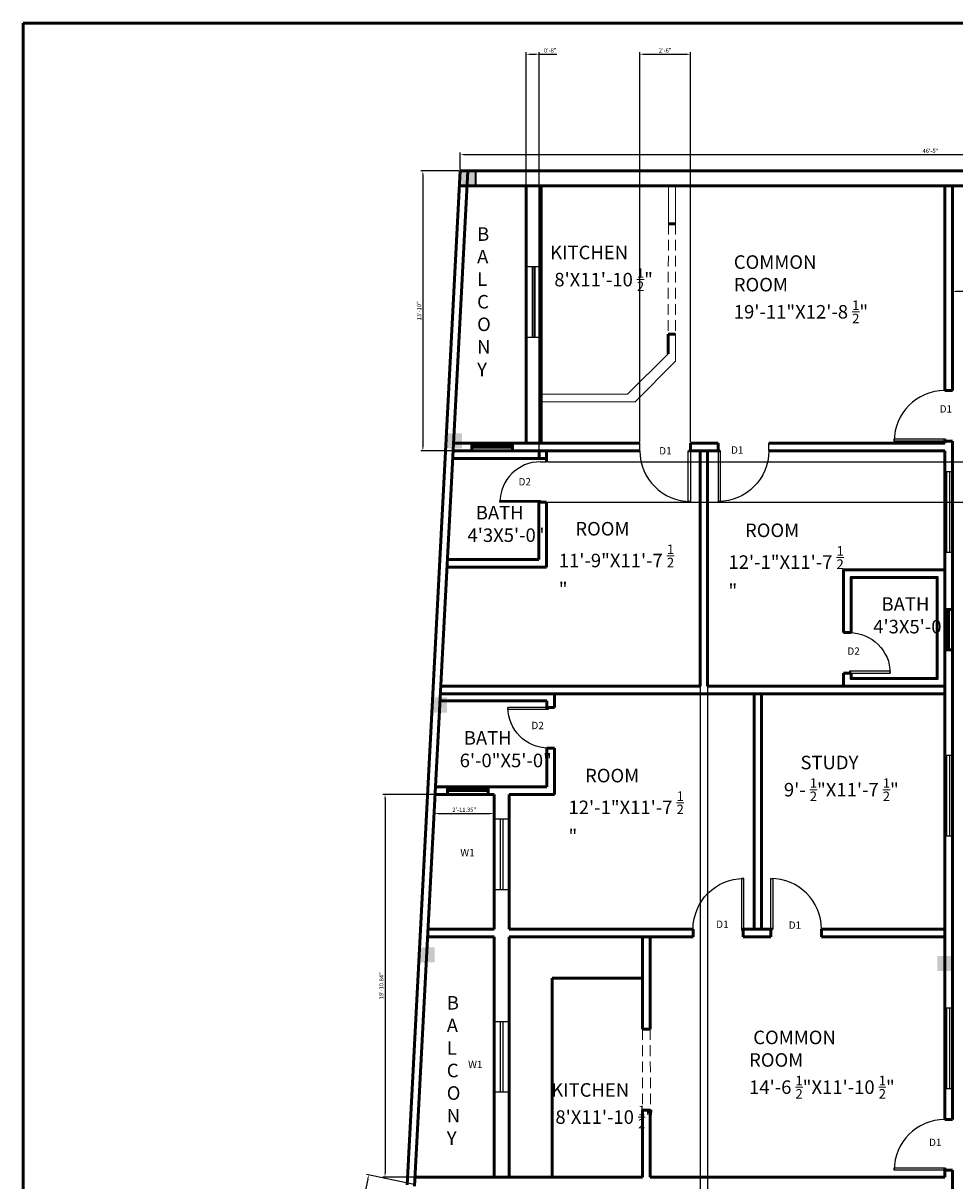
# Model space of a CAD drawing. Units: millimetres. Extents: x 1945 to 2943, y 628 to 2340.
# Tile 4 of 5: x 1945 to 2497, y 1654 to 2340. Entities that reach past the tile are written whole.
import ezdxf

# ---------------------------------------------------------------- set-up
doc = ezdxf.new("R2010")
doc.units = ezdxf.units.MM
doc.linetypes.add('DASHED', pattern=[19.05, 12.7, -6.35])
for name, color, linetype, lineweight in [('A-ANNO-DIMS', 2, 'Continuous', 18), ('A-ANNO-TEXT', 7, 'Continuous', 18), ('A-AREA-IDEN', 3, 'Continuous', 18), ('A-COLS', 1, 'Continuous', 35), ('A-DOOR', 4, 'Continuous', 25), ('A-FLOR-FIXT', 8, 'Continuous', 18), ('A-GLAZ', 4, 'Continuous', 25), ('A-WALL', 7, 'Continuous', 50), ('A-WALL-OPNG', 8, 'DASHED', 18)]:
    doc.layers.add(name, color=color, linetype=linetype, lineweight=lineweight)
doc.styles.get("Standard").update_dxf_attribs({"font": 'arial.ttf'})
doc.styles.add('YQ_DIM', font='SUPEROS.SHX', dxfattribs={"width": 0.8, "bigfont": 'HZDX.SHX'})
doc.dimstyles.new('ISO-25', dxfattribs={"dimtxt": 2.5, "dimasz": 2.5, "dimexe": 1.25, "dimexo": 0.625, "dimtad": 1, "dimlunit": 3, "dimtxsty": 'Standard', "dimcen": 2.5, "dimadec": 0, "dimazin": 0, "dimtfac": 1, "dimtmove": 0, "dimatfit": 3, "dimfxl": 1, "dimarcsym": 0})

# ---------------------------------------------------------------- blocks, each defined once
blk = doc.blocks.new('*U3')
for p, q in [((0, 0), (0, -6)), ((40, 0), (40, -6))]:
    blk.add_line(p, q)
blk.add_lwpolyline([(0, 0), (0, 40), (1.75, 40), (1.75, 0)], close=True)
blk.add_arc((0, 0), 40, 0, 90)
blk = doc.blocks.new('*D7')
at = {"layer": 'A-ANNO-DIMS', "color": 0, "lineweight": -2, "ltscale": 0.5, "transparency": 16777216}
for p, q in [((2495.1, 2172.25), (2495.1, 2182.39)), ((2633.6, 2172.25), (2633.6, 2182.39)), ((2631.1, 2181.14), (2497.6, 2181.14))]:
    blk.add_line(p, q, dxfattribs=at)
at = {"layer": 'A-ANNO-DIMS', "color": 0, "ltscale": 0.5, "transparency": 16777216}
for points in [[(2497.6, 2181.56), (2497.6, 2180.72), (2495.1, 2181.14)], [(2631.1, 2181.56), (2631.1, 2180.72), (2633.6, 2181.14)]]:
    blk.add_solid(points, dxfattribs=at)
at = {"layer": 'Defpoints', "color": 0, "ltscale": 0.5, "transparency": 16777216}
for p in [(2495.1, 2181.14), (2495.1, 2171.62), (2633.6, 2171.62)]:
    blk.add_point(p, dxfattribs=at)
at = {"layer": 'A-ANNO-DIMS', "color": 0, "ltscale": 0.5, "transparency": 16777216, "insert": (2564.35, 2183.04), "char_height": 2.5, "attachment_point": 5}
blk.add_mtext('11\'-6.5"', dxfattribs=at)
blk = doc.blocks.new('*D8')
at = {"layer": 'A-ANNO-DIMS', "color": 0, "lineweight": -2, "ltscale": 0.5, "transparency": 16777216}
for p, q in [((2202.97, 2252.62), (2180.19, 2252.62)), ((2181.44, 2250.12), (2181.44, 2089.12)), ((2198.78, 2086.62), (2180.19, 2086.62))]:
    blk.add_line(p, q, dxfattribs=at)
at = {"layer": 'A-ANNO-DIMS', "color": 0, "ltscale": 0.5, "transparency": 16777216}
for points in [[(2181.02, 2250.12), (2181.85, 2250.12), (2181.44, 2252.62)], [(2181.02, 2089.12), (2181.85, 2089.12), (2181.44, 2086.62)]]:
    blk.add_solid(points, dxfattribs=at)
at = {"layer": 'Defpoints', "color": 0, "ltscale": 0.5, "transparency": 16777216}
for p in [(2203.6, 2252.62), (2181.44, 2086.62), (2199.4, 2086.62)]:
    blk.add_point(p, dxfattribs=at)
at = {"layer": 'A-ANNO-DIMS', "color": 0, "ltscale": 0.5, "transparency": 16777216, "insert": (2179.54, 2169.62), "char_height": 2.5, "attachment_point": 5, "rotation": 90}
blk.add_mtext('13\'-10"', dxfattribs=at)
blk = doc.blocks.new('*D9')
at = {"layer": 'A-ANNO-DIMS', "color": 0, "lineweight": -2, "ltscale": 0.5, "transparency": 16777216}
for p, q in [((2188.11, 1882.96), (2157.79, 1882.96)), ((2159.04, 1880.46), (2159.04, 1658.62)), ((2176.22, 1656.12), (2157.79, 1656.12))]:
    blk.add_line(p, q, dxfattribs=at)
at = {"layer": 'A-ANNO-DIMS', "color": 0, "ltscale": 0.5, "transparency": 16777216}
for points in [[(2158.62, 1880.46), (2159.45, 1880.46), (2159.04, 1882.96)], [(2158.62, 1658.62), (2159.45, 1658.62), (2159.04, 1656.12)]]:
    blk.add_solid(points, dxfattribs=at)
at = {"layer": 'Defpoints', "color": 0, "ltscale": 0.5, "transparency": 16777216}
for p in [(2188.73, 1882.96), (2159.04, 1656.12), (2176.84, 1656.12)]:
    blk.add_point(p, dxfattribs=at)
at = {"layer": 'A-ANNO-DIMS', "color": 0, "ltscale": 0.5, "transparency": 16777216, "insert": (2157.14, 1769.54), "char_height": 2.5, "attachment_point": 5, "rotation": 90}
blk.add_mtext('18\'-10.84"', dxfattribs=at)
blk = doc.blocks.new('*D10')
at = {"layer": 'A-ANNO-DIMS', "color": 0, "lineweight": -2, "ltscale": 0.5, "transparency": 16777216}
for p, q in [((2148.79, 1654.96), (2010, 994.38)), ((2176.25, 1651.75), (2148.08, 1657.67)), ((2036.43, 986.28), (2008.27, 992.19))]:
    blk.add_line(p, q, dxfattribs=at)
at = {"layer": 'A-ANNO-DIMS', "color": 0, "ltscale": 0.5, "transparency": 16777216}
for points in [[(2148.39, 1655.05), (2149.2, 1654.88), (2149.31, 1657.41)], [(2009.6, 994.47), (2010.41, 994.3), (2009.49, 991.94)]]:
    blk.add_solid(points, dxfattribs=at)
at = {"layer": 'Defpoints', "color": 0, "ltscale": 0.5, "transparency": 16777216}
for p in [(2176.86, 1651.62), (2009.49, 991.94), (2037.04, 986.15)]:
    blk.add_point(p, dxfattribs=at)
at = {"layer": 'A-ANNO-DIMS', "color": 0, "ltscale": 0.5, "transparency": 16777216, "insert": (2077.54, 1325.06), "char_height": 2.5, "attachment_point": 5, "rotation": 78.13463}
blk.add_mtext('56\'-8"', dxfattribs=at)
blk = doc.blocks.new('*D11')
at = {"layer": 'A-ANNO-DIMS', "color": 0, "lineweight": -2, "ltscale": 0.5, "transparency": 16777216}
for p, q in [((2188.24, 1873.05), (2188.24, 1870.37)), ((2190.74, 1871.62), (2221.1, 1871.62)), ((2223.6, 1873.05), (2223.6, 1870.37))]:
    blk.add_line(p, q, dxfattribs=at)
at = {"layer": 'A-ANNO-DIMS', "color": 0, "ltscale": 0.5, "transparency": 16777216}
for points in [[(2190.74, 1872.03), (2190.74, 1871.2), (2188.24, 1871.62)], [(2221.1, 1872.03), (2221.1, 1871.2), (2223.6, 1871.62)]]:
    blk.add_solid(points, dxfattribs=at)
at = {"layer": 'Defpoints', "color": 0, "ltscale": 0.5, "transparency": 16777216}
for p in [(2188.24, 1873.68), (2223.6, 1873.68), (2223.6, 1871.62)]:
    blk.add_point(p, dxfattribs=at)
at = {"layer": 'A-ANNO-DIMS', "color": 0, "ltscale": 0.5, "transparency": 16777216, "insert": (2205.92, 1873.52), "char_height": 2.5, "attachment_point": 5}
blk.add_mtext('2\'-11.35"', dxfattribs=at)
blk = doc.blocks.new('*D17')
at = {"layer": 'A-ANNO-DIMS', "color": 0, "lineweight": -2, "transparency": 16777216}
for p, q in [((2203.6, 2253.25), (2203.6, 2263.48)), ((2206.1, 2262.23), (2758.1, 2262.23)), ((2760.6, 2253.25), (2760.6, 2263.48))]:
    blk.add_line(p, q, dxfattribs=at)
at = {"layer": 'A-ANNO-DIMS', "color": 0, "transparency": 16777216}
for points in [[(2206.1, 2262.64), (2206.1, 2261.81), (2203.6, 2262.23)], [(2758.1, 2262.64), (2758.1, 2261.81), (2760.6, 2262.23)]]:
    blk.add_solid(points, dxfattribs=at)
at = {"layer": 'Defpoints', "color": 0, "transparency": 16777216}
for p in [(2760.6, 2262.23), (2203.6, 2252.62), (2760.6, 2252.62)]:
    blk.add_point(p, dxfattribs=at)
at = {"layer": 'A-ANNO-DIMS', "color": 0, "transparency": 16777216, "insert": (2482.1, 2264.13), "char_height": 2.5, "attachment_point": 5}
blk.add_mtext('46\'-5"', dxfattribs=at)
blk = doc.blocks.new('WIN-W1')
for points in [[(0, 48), (4.5, 48), (4.5, 0), (0, 0)], [(1.29, 48), (2.82, 48), (2.82, 0), (1.29, 0)]]:
    blk.add_lwpolyline(points, close=True)
blk = doc.blocks.new('WIN-W2')
for points in [[(0, 42), (9, 42), (9, 0), (0, 0)], [(3.84, 42), (5.13, 42), (5.13, 0), (3.84, 0)]]:
    blk.add_lwpolyline(points, close=True)
blk = doc.blocks.new('*D27')
at = {"layer": 'A-ANNO-DIMS', "color": 0, "lineweight": -2, "transparency": 16777216}
for p, q in [((2309.97, 2091.75), (2309.97, 2322.97)), ((2312.47, 2321.72), (2337.47, 2321.72)), ((2339.97, 2091.75), (2339.97, 2322.97))]:
    blk.add_line(p, q, dxfattribs=at)
at = {"layer": 'A-ANNO-DIMS', "color": 0, "transparency": 16777216}
for points in [[(2312.47, 2322.14), (2312.47, 2321.3), (2309.97, 2321.72)], [(2337.47, 2322.14), (2337.47, 2321.3), (2339.97, 2321.72)]]:
    blk.add_solid(points, dxfattribs=at)
at = {"layer": 'Defpoints', "color": 0, "transparency": 16777216}
for p in [(2339.97, 2321.72), (2309.97, 2091.12), (2339.97, 2091.12)]:
    blk.add_point(p, dxfattribs=at)
at = {"layer": 'A-ANNO-DIMS', "color": 0, "transparency": 16777216, "insert": (2324.97, 2323.62), "char_height": 2.5, "attachment_point": 5}
blk.add_mtext('2\'-6"', dxfattribs=at)
blk = doc.blocks.new('*D28')
at = {"layer": 'A-ANNO-DIMS', "color": 0, "lineweight": -2, "transparency": 16777216}
for p, q in [((2255.29, 2080.13), (2830.95, 2080.13)), ((2829.7, 2058.63), (2829.7, 2077.63)), ((2255.29, 2056.13), (2830.95, 2056.13))]:
    blk.add_line(p, q, dxfattribs=at)
at = {"layer": 'A-ANNO-DIMS', "color": 0, "transparency": 16777216}
for points in [[(2829.28, 2077.63), (2830.11, 2077.63), (2829.7, 2080.13)], [(2829.28, 2058.63), (2830.11, 2058.63), (2829.7, 2056.13)]]:
    blk.add_solid(points, dxfattribs=at)
at = {"layer": 'Defpoints', "color": 0, "transparency": 16777216}
for p in [(2254.67, 2080.13), (2829.7, 2080.13), (2254.67, 2056.13)]:
    blk.add_point(p, dxfattribs=at)
at = {"layer": 'A-ANNO-DIMS', "color": 0, "transparency": 16777216, "insert": (2827.8, 2068.13), "char_height": 2.5, "attachment_point": 5, "rotation": 90}
blk.add_mtext('2\'-0"', dxfattribs=at)
blk = doc.blocks.new('*D29')
at = {"layer": 'A-ANNO-DIMS', "color": 0, "lineweight": -2, "transparency": 16777216}
for p, q in [((2242.6, 2091.75), (2242.6, 2322.97)), ((2245.1, 2321.72), (2247.9, 2321.72)), ((2250.4, 2087.25), (2250.4, 2322.97)), ((2250.4, 2321.72), (2260.8, 2321.72))]:
    blk.add_line(p, q, dxfattribs=at)
at = {"layer": 'A-ANNO-DIMS', "color": 0, "transparency": 16777216}
for points in [[(2245.1, 2322.14), (2245.1, 2321.3), (2242.6, 2321.72)], [(2247.9, 2322.14), (2247.9, 2321.3), (2250.4, 2321.72)]]:
    blk.add_solid(points, dxfattribs=at)
at = {"layer": 'Defpoints', "color": 0, "transparency": 16777216}
for p in [(2250.4, 2321.72), (2242.6, 2091.12), (2250.4, 2086.62)]:
    blk.add_point(p, dxfattribs=at)
at = {"layer": 'A-ANNO-DIMS', "color": 0, "transparency": 16777216, "insert": (2256.85, 2323.62), "char_height": 2.5, "attachment_point": 5}
blk.add_mtext('0\'-8"', dxfattribs=at)
blk = doc.blocks.new('*D30')
at = {"layer": 'A-ANNO-DIMS', "color": 0, "lineweight": -2, "transparency": 16777216}
for p, q in [((2345.6, 2086), (2345.6, 856.56)), ((2350.1, 2086), (2350.1, 856.56)), ((2343.1, 857.81), (2340.6, 857.81)), ((2345.6, 857.81), (2350.1, 857.81)), ((2352.6, 857.81), (2368.82, 857.81))]:
    blk.add_line(p, q, dxfattribs=at)
at = {"layer": 'A-ANNO-DIMS', "color": 0, "transparency": 16777216}
for points in [[(2343.1, 858.23), (2343.1, 857.39), (2345.6, 857.81)], [(2352.6, 858.23), (2352.6, 857.39), (2350.1, 857.81)]]:
    blk.add_solid(points, dxfattribs=at)
at = {"layer": 'Defpoints', "color": 0, "transparency": 16777216}
for p in [(2345.6, 2086.62), (2350.1, 2086.62), (2350.1, 857.81)]:
    blk.add_point(p, dxfattribs=at)
at = {"layer": 'A-ANNO-DIMS', "color": 0, "transparency": 16777216, "insert": (2361.96, 859.73), "char_height": 2.5, "attachment_point": 5}
blk.add_mtext('0\'-4 1/2"', dxfattribs=at)

msp = doc.modelspace()

# ---------------------------------------------------------------- hatches: boundary and pattern name
at = {"layer": 'A-COLS'}
h = msp.add_hatch(color=256, dxfattribs=at)
h.dxf.hatch_style = 1
h.paths.add_polyline_path([(2212.597, 2252.621), (2203.597, 2252.621), (2203.597, 2243.621), (2212.597, 2243.621)])
h = msp.add_hatch(color=256, dxfattribs=at)
h.dxf.hatch_style = 1
h.paths.add_polyline_path([(2212.597, 2243.621), (2212.597, 2252.621), (2203.597, 2252.621), (2203.597, 2243.621)])
h = msp.add_hatch(color=256, dxfattribs=at)
h.dxf.hatch_style = 1
h.paths.add_polyline_path([(2212.597, 2243.621), (2212.597, 2252.621), (2203.597, 2252.621), (2203.597, 2243.621)])
h = msp.add_hatch(color=256, dxfattribs=at)
h.dxf.hatch_style = 1
h.paths.add_polyline_path([(2212.597, 2243.621), (2212.597, 2252.621), (2203.597, 2252.621), (2203.597, 2243.621)])
h = msp.add_hatch(color=256, dxfattribs=at)
h.dxf.hatch_style = 1
h.paths.add_polyline_path([(2212.597, 2243.621), (2212.597, 2252.621), (2203.597, 2252.621), (2203.597, 2243.621)])
h = msp.add_hatch(color=256, dxfattribs=at)
h.dxf.hatch_style = 1
h.paths.add_polyline_path([(2212.597, 2243.621), (2212.597, 2252.621), (2203.597, 2252.621), (2203.597, 2243.621)])
h = msp.add_hatch(color=256, dxfattribs=at)
h.dxf.hatch_style = 1
h.paths.add_polyline_path([(2212.597, 2243.621), (2212.597, 2252.621), (2203.597, 2252.621), (2203.597, 2243.621)])
h = msp.add_hatch(color=256, dxfattribs=at)
h.dxf.hatch_style = 1
h.paths.add_polyline_path([(2212.597, 2243.621), (2212.597, 2252.621), (2203.597, 2252.621), (2203.597, 2243.621)])
h = msp.add_hatch(color=256, dxfattribs=at)
h.dxf.hatch_style = 1
h.paths.add_polyline_path([(2212.597, 2243.621), (2212.597, 2252.621), (2203.597, 2252.621), (2203.597, 2243.621)])
h = msp.add_hatch(color=256, dxfattribs=at)
h.dxf.hatch_style = 1
h.paths.add_polyline_path([(2212.597, 2243.621), (2212.597, 2252.621), (2203.597, 2252.621), (2203.597, 2243.621)])
h = msp.add_hatch(color=256, dxfattribs=at)
h.dxf.hatch_style = 1
h.paths.add_polyline_path([(2212.597, 2243.621), (2212.597, 2252.621), (2203.597, 2252.621), (2203.597, 2243.621)])
h = msp.add_hatch(color=256, dxfattribs=at)
h.dxf.hatch_style = 1
h.paths.add_polyline_path([(2212.597, 2243.621), (2212.597, 2252.621), (2203.597, 2252.621), (2203.597, 2243.621)])
h = msp.add_hatch(color=256, dxfattribs=at)
h.dxf.hatch_style = 1
h.paths.add_polyline_path([(2212.597, 2243.621), (2212.597, 2252.621), (2203.597, 2252.621), (2203.597, 2243.621)])
h = msp.add_hatch(color=256, dxfattribs=at)
h.dxf.hatch_style = 1
h.paths.add_polyline_path([(2212.597, 2243.621), (2212.597, 2252.621), (2203.597, 2252.621), (2203.597, 2243.621)])
h = msp.add_hatch(color=256, dxfattribs=at)
h.dxf.hatch_style = 1
h.paths.add_polyline_path([(2212.597, 2243.621), (2212.597, 2252.621), (2203.597, 2252.621), (2203.597, 2243.621)])
h = msp.add_hatch(color=256, dxfattribs=at)
h.dxf.hatch_style = 1
h.paths.add_polyline_path([(2212.597, 2243.621), (2212.597, 2252.621), (2203.597, 2252.621), (2203.597, 2243.621)])
h = msp.add_hatch(color=256, dxfattribs=at)
h.dxf.hatch_style = 1
h.paths.add_polyline_path([(2212.597, 2243.621), (2212.597, 2252.621), (2203.597, 2252.621), (2203.597, 2243.621)])
h = msp.add_hatch(color=256, dxfattribs=at)
h.dxf.hatch_style = 1
h.paths.add_polyline_path([(2212.597, 2243.621), (2212.597, 2252.621), (2203.597, 2252.621), (2203.597, 2243.621)])
h = msp.add_hatch(color=256, dxfattribs=at)
h.dxf.hatch_style = 1
h.paths.add_polyline_path([(2204.673, 2097.037), (2195.673, 2097.037), (2195.673, 2088.037), (2204.673, 2088.037)])
h = msp.add_hatch(color=256, dxfattribs=at)
h.dxf.hatch_style = 1
h.paths.add_polyline_path([(2195.693, 1940.478), (2186.693, 1940.478), (2186.693, 1931.478), (2195.693, 1931.478)])
h = msp.add_hatch(color=256, dxfattribs=at)
h.dxf.hatch_style = 1
h.paths.add_polyline_path([(2188.404, 1792.332), (2179.404, 1792.332), (2179.404, 1783.332), (2188.404, 1783.332)])
h = msp.add_hatch(color=256, dxfattribs=at)
h.dxf.hatch_style = 1
h.paths.add_polyline_path([(2495.097, 1787.253), (2486.097, 1787.253), (2486.097, 1778.253), (2495.097, 1778.253)])

# ---------------------------------------------------------------- linework, layer by layer
msp.add_lwpolyline([(2203.597, 2252.621), (2212.597, 2252.621), (2212.597, 2243.621), (2203.597, 2243.621)], close=True, dxfattribs=at)
at = {"layer": 'A-FLOR-FIXT'}
for points in [[(2326.669, 2144.192), (2302.597, 2120.192), (2251.597, 2120.192), (2251.967, 2243.621), (2326.967, 2243.621), (2326.9, 2221.255)], [(2331.097, 2243.621), (2331.097, 2221.255)], [(2247.097, 2153.851), (2247.097, 2195.851)], [(2331.097, 2155.773), (2331.097, 2139.692), (2307.097, 2115.692), (2251.597, 2115.692)]]:
    msp.add_lwpolyline(points, dxfattribs=at)
at = {"layer": 'A-WALL'}
for p, q in [((2203.597, 2252.621), (2172.098, 1651.581)), ((2208.091, 2252.386), (2176.56, 1650.732)), ((2760.597, 2252.621), (2203.597, 2252.621)), ((2751.597, 2243.621), (2203.597, 2243.621)), ((2242.597, 2243.192), (2242.597, 2091.121)), ((2251.597, 2243.192), (2251.597, 2091.121)), ((2490.597, 2243.621), (2490.597, 2122.348)), ((2495.097, 2243.621), (2495.097, 2122.348)), ((2326.9, 2221.255), (2331.097, 2221.255)), ((2326.669, 2144.192), (2326.704, 2155.773)), ((2326.704, 2155.773), (2331.097, 2155.773)), ((2495.097, 2122.348), (2490.597, 2122.348)), ((2490.597, 2093.66), (2490.597, 2091.121)), ((2309.97, 2086.621), (2199.404, 2086.621)), ((2199.404, 2086.621), (2254.668, 2086.621)), ((2309.97, 2091.121), (2199.64, 2091.121)), ((2250.404, 2086.621), (2250.404, 2082.121)), ((2254.668, 2086.621), (2254.668, 2080.13)), ((2357.406, 2086.621), (2338.92, 2086.621)), ((2356.356, 2091.121), (2339.97, 2091.121)), ((2339.97, 2091.121), (2339.97, 2086.621)), ((2345.597, 2086.621), (2345.597, 1947.121)), ((2350.097, 2086.621), (2350.097, 1947.121)), ((2356.356, 2091.121), (2356.356, 2086.621)), ((2490.597, 2091.121), (2386.356, 2091.121)), ((2490.597, 2086.621), (2386.356, 2086.621)), ((2490.597, 2092.348), (2495.097, 2092.348)), ((2490.597, 2086.621), (2490.597, 1690.225)), ((2495.097, 2092.348), (2495.097, 1690.225)), ((2199.168, 2082.121), (2254.668, 2082.121)), ((2250.168, 2057.18), (2250.168, 2022.121)), ((2250.168, 2056.13), (2254.668, 2056.13)), ((2254.668, 2056.13), (2254.668, 2017.621)), ((2254.668, 2017.621), (2195.788, 2017.621)), ((2250.168, 2022.121), (2196.024, 2022.121)), ((2430.597, 1978.881), (2435.097, 1978.864)), ((2430.597, 1954.881), (2435.097, 1954.881)), ((2490.597, 1942.621), (2191.857, 1942.621)), ((2345.597, 1947.121), (2192.093, 1947.121)), ((2259.369, 1942.621), (2259.369, 1934.461)), ((2490.597, 1947.121), (2350.097, 1947.121)), ((2377.597, 1942.621), (2377.597, 1803.121)), ((2382.097, 1942.621), (2382.097, 1803.121)), ((2191.869, 1938.462), (2254.869, 1938.462)), ((2254.869, 1938.462), (2254.869, 1933.411)), ((2254.869, 1934.461), (2259.369, 1934.461)), ((2254.869, 1910.477), (2254.869, 1887.462)), ((2254.869, 1910.477), (2259.369, 1910.477)), ((2259.369, 1910.477), (2259.369, 1882.962)), ((2254.869, 1887.462), (2188.966, 1887.462)), ((2223.597, 1882.962), (2188.731, 1882.962)), ((2223.597, 1882.962), (2223.597, 1803.121)), ((2232.597, 1882.962), (2232.597, 1803.121)), ((2259.369, 1882.962), (2232.597, 1882.962)), ((2223.597, 1798.621), (2184.31, 1798.621)), ((2223.597, 1803.121), (2184.546, 1803.121)), ((2223.597, 1798.621), (2223.597, 1656.121)), ((2341.479, 1803.121), (2232.597, 1803.121)), ((2341.479, 1798.621), (2232.597, 1798.621)), ((2232.597, 1798.621), (2232.597, 1656.121)), ((2311.597, 1798.621), (2311.597, 1743.767)), ((2311.597, 1798.621), (2311.597, 1773.951)), ((2316.097, 1798.621), (2316.097, 1743.767)), ((2341.479, 1803.121), (2341.479, 1798.621)), ((2388.537, 1803.121), (2370.051, 1803.121)), ((2371.101, 1803.121), (2371.101, 1798.621)), ((2387.487, 1798.621), (2371.101, 1798.621)), ((2387.487, 1803.121), (2387.487, 1798.621)), ((2490.597, 1803.121), (2417.487, 1803.121)), ((2417.487, 1803.121), (2417.487, 1798.621)), ((2490.597, 1798.621), (2417.487, 1798.621)), ((2311.597, 1773.951), (2257.957, 1773.951)), ((2257.957, 1773.951), (2257.957, 1656.121)), ((2311.597, 1695.768), (2311.597, 1656.121)), ((2316.097, 1695.768), (2316.097, 1656.121)), ((2490.597, 1690.225), (2495.097, 1690.225)), ((2490.597, 1661.538), (2490.597, 1656.121)), ((2311.597, 1656.121), (2176.842, 1656.121)), ((2490.597, 1656.121), (2316.097, 1656.121)), ((2490.597, 1660.225), (2495.097, 1660.225)), ((2495.097, 1660.225), (2495.097, 1545.177))]:
    msp.add_line(p, q, dxfattribs=at)
at = {"layer": 'A-WALL', "ltscale": 0.5}
for p, q in [((2311.597, 1743.767), (2316.097, 1743.767)), ((2316.276, 1695.768), (2311.597, 1695.768))]:
    msp.add_line(p, q, dxfattribs=at)
for points in [[(1944.667, 2340.145), (2943.065, 2340.145), (2943.065, 839.363), (1944.667, 839.363)], [(2234.49, 2091.121), (2234.49, 2086.621), (2210.49, 2086.621), (2210.49, 2091.121)], [(2234.49, 2089.735), (2234.49, 2088.871), (2210.49, 2088.871), (2210.49, 2089.735)], [(2490.597, 1992.581), (2495.097, 1992.581), (2495.097, 1968.581), (2490.597, 1968.581)], [(2491.984, 1992.581), (2492.847, 1992.581), (2492.847, 1968.581), (2491.984, 1968.581)], [(2220.088, 1887.462), (2220.088, 1882.962), (2196.088, 1882.962), (2196.088, 1887.462)], [(2220.088, 1886.076), (2220.088, 1885.212), (2196.088, 1885.212), (2196.088, 1886.076)]]:
    msp.add_lwpolyline(points, close=True, dxfattribs=at)
at = {"layer": 'A-WALL'}
for points in [[(2430.597, 1978.881), (2430.597, 2016.121), (2490.597, 2016.121), (2490.597, 1947.121), (2430.597, 1947.121), (2430.597, 1954.881)], [(2435.097, 1978.864), (2435.097, 2011.621), (2486.097, 2011.621), (2486.097, 1951.621), (2435.097, 1951.621), (2435.097, 1954.881)]]:
    msp.add_lwpolyline(points, dxfattribs=at)
at = {"layer": 'A-WALL-OPNG', "ltscale": 0.5}
for p, q in [((2326.9, 2221.255), (2326.704, 2155.773)), ((2331.097, 2221.255), (2331.097, 2155.773)), ((2311.597, 1743.767), (2311.597, 1695.768)), ((2316.097, 1743.767), (2316.276, 1695.768))]:
    msp.add_line(p, q, dxfattribs=at)

# ---------------------------------------------------------------- block references
at = {"layer": 'A-DOOR'}
for p, xscale, yscale, zscale, rotation in [((2490.597, 2092.348), 0.75, 0.75, 0.75, 90.00000000000003), ((2339.97, 2086.621), 0.75, 0.75, 0.75, 180), ((2356.356, 2086.621), -0.75, 0.75, 0.75, 180), ((2251.068, 2056.13), 0.6, 0.6, 0.6, 90), ((2434.197, 1954.881), -0.6, 0.6, 0.6, 270.0000000000005), ((2255.769, 1934.461), -0.6, 0.6, 0.6, 90), ((2490.597, 1660.225), 0.75, 0.75, 0.75, 90.00000000000003)]:
    msp.add_blockref('*U3', p, dxfattribs=dict(at, xscale=xscale, yscale=yscale, zscale=zscale, rotation=rotation))
at = {"layer": 'A-DOOR', "yscale": 0.75, "zscale": 0.75}
for p, xscale in [((2371.479, 1803.121), -0.75), ((2387.487, 1803.121), 0.75)]:
    msp.add_blockref('*U3', p, dxfattribs=dict(at, xscale=xscale))
at = {"layer": 'A-GLAZ'}
for name, p in [('WIN-W2', (2242.597, 2153.851)), ('WIN-W1', (2490.597, 2026.326)), ('WIN-W1', (2490.597, 1858.181)), ('WIN-W2', (2223.597, 1826.464)), ('WIN-W1', (2490.597, 1708.428)), ('WIN-W2', (2223.597, 1706.372))]:
    msp.add_blockref(name, p, dxfattribs=at)

# ---------------------------------------------------------------- texts
at = {"layer": 'A-ANNO-TEXT', "ltscale": 0.5, "char_height": 4.35068, "attachment_point": 1, "style": 'YQ_DIM'}
for s, insert in [('{\\f@Arial Unicode MS|b0|i0|c0|p34;D1}', (2487.562, 2113.657)), ('{\\f@Arial Unicode MS|b0|i0|c0|p34;D1}', (2321.405, 2088.843)), ('{\\f@Arial Unicode MS|b0|i0|c0|p34;D1}', (2363.964, 2089.299)), ('{\\f@Arial Unicode MS|b0|i0|c0|p34;D2}', (2238.105, 2070.488)), ('{\\f@Arial Unicode MS|b0|i0|c0|p34;D2}', (2432.852, 1970.07)), ('{\\f@Arial Unicode MS|b0|i0|c0|p34;D2}', (2245.709, 1925.992)), ('{\\f@Arial Unicode MS|b0|i0|c0|p34;W1}', (2203.597, 1850.606)), ('{\\f@Arial Unicode MS|b0|i0|c0|p34;D1}', (2355.176, 1808.15)), ('{\\f@Arial Unicode MS|b0|i0|c0|p34;D1}', (2398.13, 1807.667)), ('{\\f@Arial Unicode MS|b0|i0|c0|p34;W1}', (2208.25, 1725.05)), ('{\\f@Arial Unicode MS|b0|i0|c0|p34;D1}', (2481.257, 1678.878))]:
    msp.add_mtext_dynamic_manual_height_columns(s, width=7.90712, gutter_width=21.753, heights=[0], dxfattribs=dict(at, insert=insert))
at = {"layer": 'A-AREA-IDEN', "ltscale": 0.5, "attachment_point": 1, "style": 'YQ_DIM'}
for s, width, gutter_width, heights, insert, char_height in [('{\\fAcadEref|b0|i0|c0|p2;B\\f@Arial Unicode MS|b1|i1|c0|p34; A\\PL\\PC\\PO\\PN\\PY}', 12.11312, 12.5, [99.959], (2213.557, 2219.126), 8.02), ('\\A1; {\\fMicrosoft YaHei UI|b0|i0|c0|p34;KITCHEN\\P  8\'X11\'-10 \\H0.7x;\\S1/2;\\H1.42857x;"}', 67.57438, 12.5, [43.34], (2254.397, 2208.225), 8.02), ('\\A1;{\\f@Malgun Gothic|b0|i0|c0|p34;COMMON ROOM \\P19\'-11"X12\'-8 \\H0.7x;\\S1/2;\\H1.42857x;"}', 82.90028, 40.122, [0], (2365.609, 2202.535), 8.02448), ('\\A1;{\\fMicrosoft YaHei UI|b0|i0|c0|p34;  BATH\\P4\'3X5\'-0\\H1x;"}', 48.12774, 12.5, [43.34], (2207.87, 2054.007), 8.02), ('\\A1;{\\f@Malgun Gothic|b0|i0|c0|p34;    ROOM \\P11\'-9\\H1x;"X11\'-7 \\H0.7x;\\S1/2;\\H1.42857x;"}', 69.89446, 40.122, [0], (2261.941, 2044.461), 8.02448), ('\\A1;{\\f@Malgun Gothic|b0|i0|c0|p34;    ROOM \\P12\'-1\\H1x;"X11\'-7 \\H0.7x;\\S1/2;\\H1.42857x;"}', 69.89446, 40.122, [0], (2362.444, 2043.525), 8.02448), ('\\A1;{\\fMicrosoft YaHei UI|b0|i0|c0|p34;  BATH\\P4\'3X5\'-0\\H1x;"}', 48.12774, 12.5, [43.34], (2448.211, 1999.809), 8.02), ('\\A1; {\\fMicrosoft YaHei UI|b0|i0|c0|p34;BATH\\P6\'-0"X5\'-0"}', 46.26399, 12.5, [24.741], (2203.227, 1920.478), 8.02), ('\\A1;{\\f@Malgun Gothic|b0|i0|c0|p34;    STUDY\\P9\'- \\H0.7x;\\S1/2;\\H1.42857x;"X11\'-7 \\H0.7x;\\S1/2;\\H1.42857x;"}', 69.89446, 40.122, [0], (2395.293, 1905.882), 8.02448), ('\\A1;{\\f@Malgun Gothic|b0|i0|c0|p34;    ROOM \\P12\'-1\\H1x;"X11\'-7 \\H0.7x;\\S1/2;\\H1.42857x;"}', 69.89446, 40.122, [0], (2267.693, 1898.153), 8.02448), ('{\\fAcadEref|b0|i0|c0|p2;B\\f@Arial Unicode MS|b1|i1|c0|p34; A\\PL\\PC\\PO\\PN\\PY}', 12.11312, 12.5, [99.959], (2195.59, 1763.432), 8.02), ('\\A1;{\\f@Malgun Gothic|b0|i0|c0|p34; COMMON  ROOM \\P14\'-6 \\H0.7x;\\S1/2;\\H1.42857x;"X11\'-10 \\H0.7x;\\S1/2;\\H1.42857x;"}', 88.00213, 40.122, [0], (2374.671, 1742.934), 8.02448), ('\\A1; {\\fMicrosoft YaHei UI|b0|i0|c0|p34;KITCHEN\\P  8\'X11\'-10 \\H0.7x;\\S1/2;\\H1.42857x;"}', 67.57438, 12.5, [43.34], (2255.044, 1711.802), 8.02)]:
    msp.add_mtext_dynamic_manual_height_columns(s, width=width, gutter_width=gutter_width, heights=heights, dxfattribs=dict(at, insert=insert, char_height=char_height))

# ---------------------------------------------------------------- dimensions: what is measured, and where the dimension line sits
at = {"layer": 'A-ANNO-DIMS'}
for base, p1, p2, override, picture, middle in [((2250.404, 2321.721), (2242.597, 2091.121), (2250.404, 2086.621), {"dimdec": 1, "dimlfac": 1, "dimrnd": 0, "dimzin": 1, "dimdsep": 46, "dimlunit": 4, "dimfrac": 2}, '*D29', (2256.852, 2323.623)), ((2339.97, 2321.721), (2309.97, 2091.121), (2339.97, 2091.121), {"dimdec": 1, "dimlfac": 1, "dimrnd": 0, "dimzin": 1, "dimdsep": 46, "dimlunit": 4, "dimfrac": 2}, '*D27', (2324.97, 2323.623)), ((2760.597, 2262.227), (2203.597, 2252.621), (2760.597, 2252.621), {"dimclrd": 0, "dimclre": 0, "dimclrt": 0}, '*D17', (2482.097, 2264.129)), ((2350.097, 857.809), (2345.597, 2086.621), (2350.097, 2086.621), {"dimdec": 1, "dimlfac": 1, "dimrnd": 0, "dimzin": 1, "dimdsep": 46, "dimlunit": 4, "dimfrac": 2}, '*D30', (2361.958, 859.727))]:
    dim = msp.add_linear_dim(base=base, p1=p1, p2=p2, dimstyle='ISO-25', override=override, dxfattribs=at)
    dim.commit()
    dim.dimension.update_dxf_attribs({"geometry": picture, "text_midpoint": middle})
at = {"layer": 'A-ANNO-DIMS', "ltscale": 0.5}
for base, p1, p2, picture, middle in [((2181.437, 2086.621), (2203.597, 2252.621), (2199.404, 2086.621), '*D8', (2179.535, 2169.621)), ((2159.036, 1656.121), (2188.731, 1882.962), (2176.842, 1656.121), '*D9', (2157.135, 1769.542))]:
    dim = msp.add_linear_dim(base=base, p1=p1, p2=p2, angle=90, dimstyle='ISO-25', override={"dimclrd": 0, "dimclre": 0, "dimclrt": 0}, dxfattribs=at)
    dim.commit()
    dim.dimension.update_dxf_attribs({"geometry": picture, "text_midpoint": middle})
for base, p1, p2, picture, middle in [((2495.097, 2181.14), (2633.597, 2171.621), (2495.097, 2171.621), '*D7', (2564.347, 2183.042)), ((2223.597, 1871.616), (2188.244, 1873.677), (2223.597, 1873.677), '*D11', (2205.921, 1873.518))]:
    dim = msp.add_linear_dim(base=base, p1=p1, p2=p2, dimstyle='ISO-25', override={"dimclrd": 0, "dimclre": 0, "dimclrt": 0}, dxfattribs=at)
    dim.commit()
    dim.dimension.update_dxf_attribs({"geometry": picture, "text_midpoint": middle})
at = {"layer": 'A-ANNO-DIMS'}
dim = msp.add_linear_dim(base=(2829.697, 2080.13), p1=(2254.668, 2056.13), p2=(2254.668, 2080.13), angle=90, dimstyle='ISO-25', override={"dimdec": 1, "dimlfac": 1, "dimrnd": 0, "dimzin": 1, "dimdsep": 46, "dimlunit": 4, "dimfrac": 2}, dxfattribs=at)
dim.commit()
dim.dimension.update_dxf_attribs({"geometry": '*D28', "text_midpoint": (2827.796, 2068.13)})
at = {"layer": 'A-ANNO-DIMS', "ltscale": 0.5}
dim = msp.add_aligned_dim(p1=(2176.859, 1651.621), p2=(2037.041, 986.148), distance=-28.153, dimstyle='ISO-25', override={"dimclrd": 0, "dimclre": 0, "dimclrt": 0}, dxfattribs=at)
dim.commit()
dim.dimension.update_dxf_attribs({"geometry": '*D10', "text_midpoint": (2077.538, 1325.064)})

doc.saveas('drawing.dxf')
